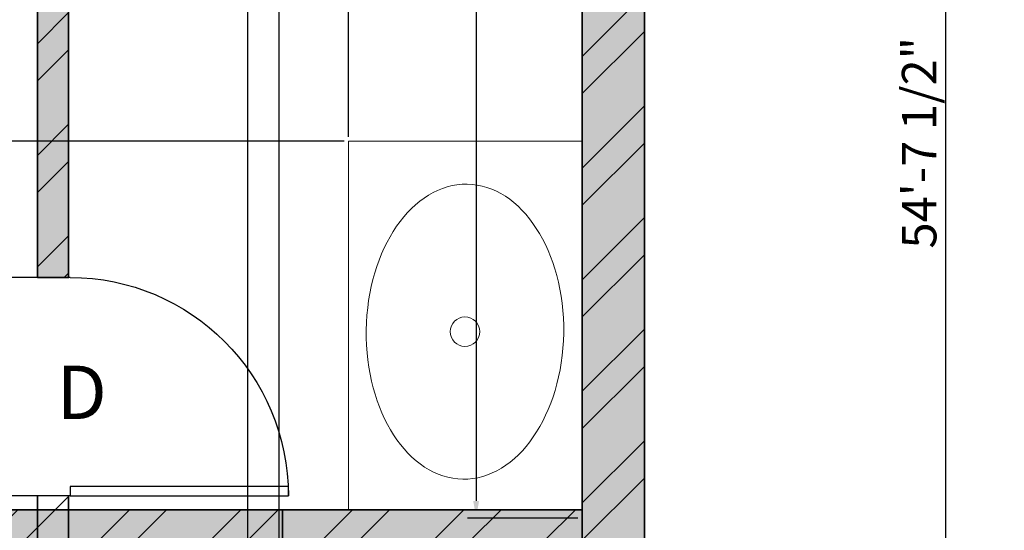
# Model space of a CAD drawing. Units: inches. Extents: x 1804 to 3296, y 909 to 2477.
# Tile 15 of 31: x 2235 to 2378, y 1410 to 1484. Entities that reach past the tile are written whole.
import ezdxf

# ---------------------------------------------------------------- set-up
doc = ezdxf.new("R2010")
doc.units = ezdxf.units.IN
for name, color, linetype, lineweight in [('A-ANNO-DIMS', 2, 'Continuous', 18), ('A-ANNO-TTLB', 156, 'Continuous', 35), ('A-FLOR-FIXT', 9, 'Continuous', 18), ('A-WALL-PATT', 10, 'Continuous', 13), ('DOOR', 30, 'Continuous', 25), ('TEXT', 190, 'Continuous', 18), ('WALL', 10, 'Continuous', 35)]:
    doc.layers.add(name, color=color, linetype=linetype, lineweight=lineweight)
doc.styles.get("Standard").update_dxf_attribs({"font": 'arial.ttf'})
doc.dimstyles.new('ISO-25', dxfattribs={"dimtxt": 5, "dimasz": 2.5, "dimexe": 1.25, "dimexo": 0.625, "dimtad": 1, "dimdec": 0, "dimlunit": 4, "dimtxsty": 'Standard', "dimcen": 2.5, "dimadec": 0, "dimazin": 0, "dimtfac": 1, "dimtdec": 0, "dimtmove": 0, "dimatfit": 3, "dimfxl": 1, "dimarcsym": 0})

# ---------------------------------------------------------------- blocks, each defined once
blk = doc.blocks.new('*U2')
for p, q in [((0, 0), (0, -6)), ((40, 0), (40, -6))]:
    blk.add_line(p, q)
blk.add_lwpolyline([(0, 0), (0, 40), (1.75, 40), (1.75, 0)], close=True)
blk.add_arc((0, 0), 40, 0, 90)
blk = doc.blocks.new('*D13')
at = {"layer": 'A-ANNO-DIMS', "color": 0, "lineweight": -2, "transparency": 16777216}
for p, q in [((2315.91, 1586.42), (2299.9, 1586.42)), ((2301.15, 1583.92), (2301.15, 1413.85)), ((2315.91, 1411.35), (2299.9, 1411.35))]:
    blk.add_line(p, q, dxfattribs=at)
at = {"layer": 'A-ANNO-DIMS', "color": 0, "lineweight": 100, "transparency": 16777216}
for points in [[(2300.73, 1583.92), (2301.57, 1583.92), (2301.15, 1586.42)], [(2300.73, 1413.85), (2301.57, 1413.85), (2301.15, 1411.35)]]:
    blk.add_solid(points, dxfattribs=at)
at = {"layer": 'Defpoints', "color": 0, "lineweight": 100, "transparency": 16777216}
for p in [(2316.54, 1586.42), (2301.15, 1411.35), (2316.54, 1411.35)]:
    blk.add_point(p, dxfattribs=at)
at = {"layer": 'A-ANNO-DIMS', "color": 0, "transparency": 16777216, "insert": (2298.02, 1498.89), "char_height": 5, "attachment_point": 5, "rotation": 90}
blk.add_mtext('14\'-7"', dxfattribs=at)
blk = doc.blocks.new('*D53')
at = {"layer": 'A-ANNO-DIMS', "color": 0, "lineweight": -2, "transparency": 16777216}
for p, q in [((2326.16, 1793.38), (2370.49, 1793.38)), ((2369.24, 1140.57), (2369.24, 1790.88)), ((2326.16, 1138.07), (2370.49, 1138.07))]:
    blk.add_line(p, q, dxfattribs=at)
at = {"layer": 'A-ANNO-DIMS', "color": 0, "lineweight": 100, "transparency": 16777216}
for points in [[(2368.82, 1790.88), (2369.65, 1790.88), (2369.24, 1793.38)], [(2368.82, 1140.57), (2369.65, 1140.57), (2369.24, 1138.07)]]:
    blk.add_solid(points, dxfattribs=at)
at = {"layer": 'Defpoints', "color": 0, "lineweight": 100, "transparency": 16777216}
for p in [(2325.54, 1793.38), (2369.24, 1793.38), (2325.54, 1138.07)]:
    blk.add_point(p, dxfattribs=at)
at = {"layer": 'A-ANNO-DIMS', "color": 0, "transparency": 16777216, "insert": (2366.03, 1465.72), "char_height": 5, "attachment_point": 5, "rotation": 90}
blk.add_mtext('54\'-7 1/2"', dxfattribs=at)
blk = doc.blocks.new('*D56')
at = {"layer": 'A-ANNO-DIMS', "color": 0, "lineweight": -2, "transparency": 16777216}
for p, q in [((2180.87, 1680.42), (2180.87, 975.89)), ((2268, 1680.42), (2268, 975.89)), ((2183.37, 977.14), (2265.5, 977.14))]:
    blk.add_line(p, q, dxfattribs=at)
at = {"layer": 'A-ANNO-DIMS', "color": 0, "lineweight": 100, "transparency": 16777216}
for points in [[(2183.37, 977.56), (2183.37, 976.72), (2180.87, 977.14)], [(2265.5, 977.56), (2265.5, 976.72), (2268, 977.14)]]:
    blk.add_solid(points, dxfattribs=at)
at = {"layer": 'Defpoints', "color": 0, "lineweight": 100, "transparency": 16777216}
for p in [(2180.87, 1681.04), (2268, 1681.04), (2268, 977.14)]:
    blk.add_point(p, dxfattribs=at)
at = {"layer": 'A-ANNO-DIMS', "color": 0, "transparency": 16777216, "insert": (2224.44, 980.32), "char_height": 5, "attachment_point": 5}
blk.add_mtext('7\'-3"', dxfattribs=at)
blk = doc.blocks.new('*D64')
at = {"layer": 'A-ANNO-DIMS', "color": 0, "lineweight": -2, "transparency": 16777216}
for p, q in [((2241.43, 1446.21), (1880.63, 1446.21)), ((1881.88, 1417.08), (1881.88, 1443.71)), ((2241.43, 1414.58), (1880.63, 1414.58))]:
    blk.add_line(p, q, dxfattribs=at)
at = {"layer": 'A-ANNO-DIMS', "color": 0, "lineweight": 100, "transparency": 16777216}
for points in [[(1881.47, 1443.71), (1882.3, 1443.71), (1881.88, 1446.21)], [(1881.47, 1417.08), (1882.3, 1417.08), (1881.88, 1414.58)]]:
    blk.add_solid(points, dxfattribs=at)
at = {"layer": 'Defpoints', "color": 0, "lineweight": 100, "transparency": 16777216}
for p in [(1881.88, 1446.21), (2242.06, 1446.21), (2242.06, 1414.58)]:
    blk.add_point(p, dxfattribs=at)
at = {"layer": 'A-ANNO-DIMS', "color": 0, "transparency": 16777216, "insert": (1878.67, 1430.39), "char_height": 5, "attachment_point": 5, "rotation": 90}
blk.add_mtext('2\'-7 1/2"', dxfattribs=at)
blk = doc.blocks.new('*D65')
at = {"layer": 'A-ANNO-DIMS', "color": 0, "lineweight": -2, "transparency": 16777216}
for p, q in [((2282.65, 1466.57), (2282.65, 1874.99)), ((2316.54, 1466.57), (2316.54, 1874.99)), ((2285.15, 1873.74), (2314.04, 1873.74))]:
    blk.add_line(p, q, dxfattribs=at)
at = {"layer": 'A-ANNO-DIMS', "color": 0, "lineweight": 100, "transparency": 16777216}
for points in [[(2285.15, 1874.15), (2285.15, 1873.32), (2282.65, 1873.74)], [(2314.04, 1874.15), (2314.04, 1873.32), (2316.54, 1873.74)]]:
    blk.add_solid(points, dxfattribs=at)
at = {"layer": 'Defpoints', "color": 0, "lineweight": 100, "transparency": 16777216}
for p in [(2316.54, 1873.74), (2282.65, 1465.94), (2316.54, 1465.94)]:
    blk.add_point(p, dxfattribs=at)
at = {"layer": 'A-ANNO-DIMS', "color": 0, "transparency": 16777216, "insert": (2299.6, 1876.91), "char_height": 5, "attachment_point": 5}
blk.add_mtext('2\'-10"', dxfattribs=at)
blk = doc.blocks.new('*D66')
at = {"layer": 'A-ANNO-DIMS', "color": 0, "lineweight": -2, "transparency": 16777216}
for p, q in [((2282.03, 1465.94), (1880.63, 1465.94)), ((1881.88, 1415.06), (1881.88, 1463.44)), ((2282.03, 1412.56), (1880.63, 1412.56))]:
    blk.add_line(p, q, dxfattribs=at)
at = {"layer": 'A-ANNO-DIMS', "color": 0, "lineweight": 100, "transparency": 16777216}
for points in [[(1881.47, 1463.44), (1882.3, 1463.44), (1881.88, 1465.94)], [(1881.47, 1415.06), (1882.3, 1415.06), (1881.88, 1412.56)]]:
    blk.add_solid(points, dxfattribs=at)
at = {"layer": 'Defpoints', "color": 0, "lineweight": 100, "transparency": 16777216}
for p in [(1881.88, 1465.94), (2282.65, 1465.94), (2282.65, 1412.56)]:
    blk.add_point(p, dxfattribs=at)
at = {"layer": 'A-ANNO-DIMS', "color": 0, "transparency": 16777216, "insert": (1878.67, 1439.25), "char_height": 5, "attachment_point": 5, "rotation": 90}
blk.add_mtext('4\'-5 1/2"', dxfattribs=at)
blk = doc.blocks.new('*D73')
at = {"layer": 'A-ANNO-DIMS', "color": 0, "lineweight": -2, "transparency": 16777216}
for p, q in [((2272.59, 1272.26), (2272.59, 1874.99)), ((2316.54, 1272.26), (2316.54, 1874.99)), ((2275.09, 1873.74), (2314.04, 1873.74))]:
    blk.add_line(p, q, dxfattribs=at)
at = {"layer": 'A-ANNO-DIMS', "color": 0, "lineweight": 100, "transparency": 16777216}
for points in [[(2275.09, 1874.15), (2275.09, 1873.32), (2272.59, 1873.74)], [(2314.04, 1874.15), (2314.04, 1873.32), (2316.54, 1873.74)]]:
    blk.add_solid(points, dxfattribs=at)
at = {"layer": 'Defpoints', "color": 0, "lineweight": 100, "transparency": 16777216}
for p in [(2316.54, 1873.74), (2272.59, 1271.63), (2316.54, 1271.63)]:
    blk.add_point(p, dxfattribs=at)
at = {"layer": 'A-ANNO-DIMS', "color": 0, "transparency": 16777216, "insert": (2294.56, 1876.92), "char_height": 5, "attachment_point": 5}
blk.add_mtext('3\'-8"', dxfattribs=at)

msp = doc.modelspace()

# ---------------------------------------------------------------- hatches: boundary and pattern name
at = {"layer": 'A-ANNO-TTLB'}
h = msp.add_hatch(color=256, dxfattribs=at)
h.dxf.hatch_style = 1
h.paths.add_polyline_path([(3294.53, 2476.54), (1803.79, 2476.54), (1805.43, 909.47), (3296.17, 909.47)])
h.paths.add_polyline_path([(1811, 914.33), (1812.79, 2467.54), (3285.53, 2467.54), (3283.74, 914.33)], flags=16)
h.paths.add_polyline_path([(1925.58, 1062.77), (1925.58, 1138.07), (1925.58, 1539.88), (1925.58, 1793.38), (1925.58, 1830.04), (2325.54, 1830.04), (2325.54, 1793.38), (2325.54, 1586.42), (2325.54, 1138.07), (2325.54, 1062.77)], flags=0)
h.paths.add_polyline_path([(1997.22, 1029.4), (2008.85, 1037.96), (2008.85, 1020.84)], flags=0)
h.paths.add_polyline_path([(1934.58, 1138.07), (1934.58, 1147.07), (2078.77, 1147.07), (2078.77, 1138.07), (2060.94, 1138.07)], flags=0)
h.paths.add_polyline_path([(1944.35, 1138.07), (1944.35, 1147.07), (2056.05, 1147.07), (2056.05, 1138.07)], flags=0)
h.paths.add_polyline_path([(2222.24, 1037.96), (2233.87, 1029.4), (2222.24, 1020.84)], flags=0)
h.paths.add_polyline_path([(2061.94, 1139.07), (2061.94, 1146.07), (2077.77, 1146.07), (2077.77, 1139.07)], flags=0)
h.paths.add_polyline_path([(2149.58, 1138.07), (2149.58, 1269.44), (2158.58, 1269.44), (2158.58, 1326.69), (2149.58, 1326.69), (2149.58, 1340.94), (2139.6, 1340.94), (2139.6, 1434.25), (2149.58, 1434.25), (2149.58, 1447.36), (2158.58, 1447.36), (2158.58, 1423.87), (2158.58, 1408.06), (2198.46, 1408.06), (2198.46, 1412.56), (2282.65, 1412.56), (2282.65, 1465.94), (2316.54, 1465.94), (2316.54, 1590.92), (2192.86, 1590.92), (2192.86, 1595.3), (2291.17, 1595.3), (2291.17, 1590.92), (2316.54, 1590.92), (2316.54, 1784.38), (2300.24, 1784.38), (2300.24, 1757.47), (2268, 1757.47), (2268, 1681.04), (2180.87, 1681.04), (2180.87, 1757.47), (2148.63, 1757.47), (2148.63, 1784.38), (2119.08, 1784.38), (2119.08, 1585.58), (2114.58, 1585.58), (2114.58, 1784.38), (2064.11, 1784.38), (2046.28, 1784.38), (2046.28, 1760.38), (1958.58, 1760.38), (1958.58, 1664.38), (1934.58, 1664.38), (1934.58, 1784.38), (1934.58, 1793.38), (2046.28, 1793.38), (2064.11, 1793.38), (2119.08, 1793.38), (2230.78, 1793.38), (2230.78, 1784.38), (2268, 1784.38), (2300.24, 1784.38), (2316.54, 1784.38), (2316.54, 1590.92), (2316.54, 1373.73), (2316.54, 1138.07)], flags=0)
h.paths.add_polyline_path([(2209.19, 1166.63), (2209.19, 1175.63), (2158.58, 1175.63), (2209.19, 1223.63), (2209.19, 1231.63), (2183.88, 1231.63), (2183.88, 1301.66), (2242.59, 1301.66), (2242.59, 1326.69), (2316.54, 1326.69), (2272.59, 1271.63), (2272.59, 1223.63), (2316.54, 1175.63), (2272.59, 1175.63), (2272.59, 1166.63)], flags=0)
h.paths.add_polyline_path([(1947.77, 1345.22), (1947.77, 1457.48), (1991.2, 1457.48), (1991.2, 1451.7), (1991.2, 1352.18), (1991.2, 1345.22)], flags=0)
h.paths.add_polyline_path([(2209.19, 1271.63), (2262.59, 1271.63), (2262.59, 1311.85), (2272.59, 1301.66), (2272.59, 1271.63), (2269.92, 1269.63), (2270.59, 1269.63), (2270.59, 1225.63), (2211.19, 1225.63), (2211.19, 1269.63), (2211.86, 1269.63)], flags=0)
h.paths.add_polyline_path([(2000.34, 1378.21), (2000.34, 1429.71), (2025.22, 1429.71), (2025.22, 1378.21)], flags=0)
h.paths.add_polyline_path([(2001.34, 1379.21), (2001.34, 1428.71), (2024.22, 1428.71), (2024.22, 1379.21)], flags=0)
h.paths.add_polyline_path([(2012.34, 1390.21), (2012.34, 1417.71), (2013.22, 1417.71), (2013.22, 1390.21)], flags=0)
h.paths.add_polyline_path([(2237.56, 1331.19), (2237.56, 1340.18), (2238.62, 1340.18), (2238.62, 1386.84), (2241.04, 1386.84), (2242.06, 1386.84), (2242.06, 1408.06), (2316.54, 1331.19)], flags=0)
h.paths.add_polyline_path([(1953.73, 1464.35), (1953.73, 1498.59), (1981.74, 1498.59), (1981.74, 1464.35)], flags=0)
h.paths.add_polyline_path([(1987.63, 1462.08), (1987.63, 1500.95), (2104.07, 1500.95), (2104.07, 1462.08), (2099.27, 1462.08), (1993.6, 1462.08)], flags=0)
h.paths.add_polyline_path([(1956.06, 1481.47, -1), (1979.41, 1481.47, -1)], flags=0)
edge = h.paths.add_edge_path(flags=0)
edge.add_ellipse((2299.53, 1438.37), major_axis=(0.31, 21.36), ratio=0.670333, start_angle=0, end_angle=360)
h.paths.add_polyline_path([(2297.39, 1438.37, -1), (2301.67, 1438.37, -1)], flags=0)
h.paths.add_polyline_path([(2591.54, 1163.23), (2591.54, 1179.38), (2591.54, 1379.68), (2591.54, 1395.84), (2734.5, 1395.84), (2734.5, 1379.68), (2734.5, 1179.38), (2734.5, 1163.23)], flags=0)
h.paths.add_polyline_path([(2592.54, 1164.23), (2592.54, 1166.23), (2733.5, 1166.23), (2733.5, 1164.23)], flags=0)
h.paths.add_polyline_path([(2592.54, 1180.38), (2592.54, 1378.68), (2733.5, 1378.68), (2733.5, 1180.38)], flags=0)
h.paths.add_polyline_path([(2593.54, 1181.38), (2593.54, 1377.68), (2732.5, 1377.68), (2732.5, 1181.38)], flags=0)
h.paths.add_polyline_path([(2594.54, 1182.38), (2594.54, 1376.68), (2731.5, 1376.68), (2731.5, 1182.38)], flags=0)
h.paths.add_polyline_path([(1936.95, 1697.46), (1936.95, 1736.46), (1955.41, 1736.46), (1955.41, 1697.46)], flags=0)
h.paths.add_polyline_path([(1938.48, 1718.36), (1938.48, 1734.92), (1953.65, 1734.92), (1953.65, 1718.36)], flags=0)
h.paths.add_polyline_path([(1944.75, 1726.64, -1), (1947.37, 1726.64, -1)], flags=0)
h.paths.add_polyline_path([(2592.54, 1394.84), (2733.5, 1394.84), (2733.5, 1392.84), (2592.54, 1392.84)], flags=0)
h.paths.add_polyline_path([(1976.61, 1762.5), (1976.61, 1781.44), (2012.79, 1781.44), (2012.79, 1762.5)], flags=0)
h.paths.add_polyline_path([(1979.57, 1771.97, -1), (1991.39, 1771.97, -1)], flags=0)
h.paths.add_polyline_path([(1995.36, 1771.97, -1), (2007.18, 1771.97, -1)], flags=0)
h.paths.add_polyline_path([(2251.51, 1744.53), (2268, 1730.05), (2251.51, 1730.05)], flags=0)
h.paths.add_polyline_path([(2047.28, 1785.38), (2047.28, 1792.38), (2063.11, 1792.38), (2063.11, 1785.38)], flags=0)
h.paths.add_polyline_path([(2155.08, 1770.92, -1), (2174.42, 1770.92, -1)], flags=0)
h.paths.add_polyline_path([(2188.59, 1758.27), (2188.59, 1772.81), (2222.3, 1772.81), (2222.3, 1758.27)], flags=0)
h.paths.add_polyline_path([(2223.97, 1758.27), (2223.97, 1772.81), (2257.68, 1772.81), (2257.68, 1758.27)], flags=0)
h.paths.add_polyline_path([(2274.45, 1770.92, -1), (2293.8, 1770.92, -1)], flags=0)
h.paths.add_polyline_path([(2591.54, 1582.09), (2591.54, 1782.39), (2734.5, 1782.39), (2734.5, 1582.09)], flags=0)
h.paths.add_polyline_path([(2592.54, 1583.09), (2592.54, 1781.39), (2733.5, 1781.39), (2733.5, 1583.09)], flags=0)
h.paths.add_polyline_path([(2593.54, 1584.09), (2593.54, 1780.39), (2732.5, 1780.39), (2732.5, 1584.09)], flags=0)
h.paths.add_polyline_path([(2594.54, 1585.09), (2594.54, 1779.39), (2731.5, 1779.39), (2731.5, 1585.09)], flags=0)
h.paths.add_polyline_path([(1922.17, 1978.79), (1922.17, 2295.08), (1922.17, 2296.08), (2115.67, 2296.08), (2115.67, 2384.31), (2115.67, 2385.31), (2322.12, 2385.31), (2323.12, 2385.31), (2323.12, 1979.79), (2323.12, 1978.79), (1923.17, 1978.79)], flags=0)
h.paths.add_polyline_path([(1922.17, 1978.79), (1922.17, 2051.31), (1922.17, 2214.86), (1922.17, 2296.08), (2115.67, 2296.08), (2115.67, 2385.31), (2323.12, 2385.31), (2323.12, 2280.42), (2323.12, 1978.79), (2115.67, 1978.79)], flags=0)
h.paths.add_polyline_path([(1923.17, 1979.79), (1923.17, 2050.31), (2115.67, 2050.31), (2115.67, 2051.31), (1923.17, 2051.31), (1923.17, 2213.86), (1923.17, 2214.86), (1923.17, 2295.08), (1990.02, 2295.08), (1990.02, 2214.86), (1991.02, 2214.86), (1991.02, 2295.08), (2115.67, 2295.08), (2115.67, 1979.79), (2116.67, 1979.79), (2116.67, 2304.18), (2116.67, 2384.31), (2322.12, 2384.31), (2322.12, 2280.42), (2322.12, 1979.79), (2115.67, 1979.79)], flags=0)
h.paths.add_polyline_path([(2972.46, 1192.5), (2972.46, 1196.92), (2995.47, 1196.92), (2995.47, 1255.47), (2995.09, 1255.47), (2987.42, 1249.39), (2980.08, 1255.47), (2978.05, 1255.47), (2978.05, 1257.24), (2995.47, 1257.24), (2995.47, 1261.58), (3015.37, 1261.58), (3015.37, 1333.28), (3015.37, 1414.4), (3032.82, 1414.4), (3032.82, 1333.28), (3032.82, 1261.58), (3052.66, 1261.58), (3052.66, 1255.47), (3079.86, 1255.47), (3078.72, 1254.57), (3081.47, 1252.29), (3078.56, 1249.99), (3075.81, 1252.26), (3072.57, 1249.69), (3070.36, 1251.52), (3067.67, 1249.39), (3060.34, 1255.47), (3052.66, 1255.47), (3052.66, 1196.92), (3054.58, 1196.92), (3074, 1196.92), (3074, 1192.5), (3052.66, 1192.5), (2995.47, 1192.5)], flags=0)
h.paths.add_polyline_path([(2490.75, 1979.27), (2490.75, 1980.27), (2596.87, 1980.27), (2596.87, 2051.8), (2596.87, 2052.8), (2596.87, 2216.35), (2596.87, 2297.57), (2717.32, 2297.57), (2710.57, 2305.62), (2724.07, 2305.62), (2717.32, 2297.57), (2782.37, 2297.57), (2782.37, 2395.8), (3006.82, 2395.8), (3006.82, 1981.27), (3093.73, 1981.27), (3093.73, 1980.27), (3047.51, 1980.27), (3046.37, 1979.37), (3049.11, 1977.1), (3046.2, 1974.79), (3043.46, 1977.07), (3040.21, 1974.49), (3038, 1976.32), (3035.32, 1974.2), (3027.98, 1980.27), (2871.83, 1980.27), (2871.83, 1981.27), (2791.37, 1981.27), (2791.37, 2050.8), (2597.87, 2050.8), (2597.87, 1980.27), (2597.87, 1979.27), (2546.27, 1979.27), (2545.12, 1978.37), (2547.87, 1976.1), (2544.96, 1973.79), (2542.22, 1976.07), (2538.97, 1973.49), (2536.76, 1975.32), (2534.07, 1973.2), (2526.74, 1979.27)], flags=0)
h.paths.add_polyline_path([(2597.87, 2051.8), (2606.87, 2051.8), (2606.87, 2258.39), (2597.87, 2258.39), (2597.87, 2296.57), (2606.87, 2296.57), (2606.87, 2262.39), (2782.37, 2262.39), (2782.37, 2296.57), (2790.37, 2296.57), (2790.37, 2262.39), (2791.37, 2262.39), (2791.37, 2305.67), (2791.37, 2385.8), (2996.82, 2385.8), (2996.82, 2339.85), (3006.82, 2339.85), (3006.82, 2250.12), (2997.82, 2250.12), (2997.82, 1981.27), (2996.82, 1981.27), (2872.83, 1981.27), (2872.83, 1991.8), (2871.83, 1991.8), (2871.83, 2050.8), (2790.37, 2050.8), (2597.87, 2050.8)], flags=0)
h.paths.add_polyline_path([(2179.93, 2153.92), (2179.93, 2353.97), (2259.98, 2353.97), (2259.98, 2153.92)], flags=0)
h.paths.add_polyline_path([(2180.93, 2154.92), (2180.93, 2352.97), (2258.98, 2352.97), (2258.98, 2154.92)], flags=0)
h.paths.add_polyline_path([(2960.87, 1608.49), (2960.87, 1753.62), (3070.9, 1753.62), (3070.9, 1608.49)], flags=0)
h.paths.add_polyline_path([(2961.87, 1609.49), (2961.87, 1752.62), (3069.9, 1752.62), (3069.9, 1609.49)], flags=0)
h.paths.add_polyline_path([(2962.87, 1610.49), (2962.87, 1751.62), (3068.9, 1751.62), (3068.9, 1610.49)], flags=0)
h.paths.add_polyline_path([(2963.87, 1611.49), (2963.87, 1750.62), (3067.9, 1750.62), (3067.9, 1611.49)], flags=0)
h.paths.add_polyline_path([(2782.37, 2051.8), (2782.37, 2216.32), (2791.37, 2216.32), (2791.37, 2051.8), (2872.83, 2051.8), (2872.83, 2068.56), (2884.67, 2068.56), (2884.67, 2085.33), (2896.51, 2085.33), (2896.51, 2102.09), (2908.36, 2102.09), (2908.36, 2118.85), (2920.2, 2118.85), (2920.2, 2135.62), (2932.05, 2135.62), (2932.05, 2145.3), (2925.08, 2145.3), (2925.08, 2203.2), (2996.82, 2203.2), (2996.82, 2145.3), (2953.82, 2145.3), (2872.83, 2051.8), (2790.37, 2051.8)], flags=0)
h.paths.add_polyline_path([(2717.32, 2238.65), (2710.57, 2246.7), (2724.07, 2246.7)], flags=0)
h.paths.add_polyline_path([(2003.09, 1122.79), (2017.16, 1122.79), (2017.16, 1138.74), (2003.09, 1138.74)], flags=8)
h.paths.add_polyline_path([(2174.76, 1792.72), (2188.83, 1792.72), (2188.83, 1808.66), (2174.76, 1808.66)], flags=8)
h.paths.add_polyline_path([(1987.95, 1792.51), (2002.02, 1792.51), (2002.02, 1808.45), (1987.95, 1808.45)], flags=8)
h.paths.add_polyline_path([(2148.79, 1289.26), (2160.46, 1289.26), (2160.46, 1305.2), (2148.79, 1305.2)], flags=8)
h.paths.add_polyline_path([(2115.36, 1133.57), (2127.04, 1133.57), (2127.04, 1149.51), (2115.36, 1149.51)], flags=8)
h.paths.add_polyline_path([(2237.58, 1421.48), (2249.25, 1421.48), (2249.25, 1437.43), (2237.58, 1437.43)], flags=8)
h.paths.add_polyline_path([(2134.99, 1584.32), (2146.66, 1584.32), (2146.66, 1600.26), (2134.99, 1600.26)], flags=8)
h.paths.add_polyline_path([(2101.95, 1557.31), (2113.62, 1557.31), (2113.62, 1573.25), (2101.95, 1573.25)], flags=8)
h.paths.add_polyline_path([(2937.85, 1156.77), (3120.41, 1156.77), (3120.41, 1185.72), (2937.85, 1185.72)], flags=8)
h.paths.add_polyline_path([(2980.71, 1786.71), (3050.06, 1786.71), (3050.06, 1802.66), (2980.71, 1802.66)], flags=8)
h.paths.add_polyline_path([(2869.28, 1661.96), (2938.62, 1661.96), (2938.62, 1690.8), (2869.28, 1690.8)], flags=8)
h.paths.add_polyline_path([(3092.27, 1674.86), (3161.62, 1674.86), (3161.62, 1690.8), (3092.27, 1690.8)], flags=8)
h.paths.add_polyline_path([(2980.71, 1674.86), (3050.06, 1674.86), (3050.06, 1690.8), (2980.71, 1690.8)], flags=8)
h.paths.add_polyline_path([(2649.07, 1678.23), (2674.53, 1678.23), (2674.53, 1714.76), (2649.07, 1714.76)], flags=8)
h.paths.add_polyline_path([(2530.84, 1981.63), (2549.13, 1981.63), (2549.13, 1997.57), (2530.84, 1997.57)], flags=8)
h.paths.add_polyline_path([(3031.29, 1981.77), (3049.58, 1981.77), (3049.58, 1997.71), (3031.29, 1997.71)], flags=8)
h.paths.add_polyline_path([(2715.38, 1911.9), (2851.54, 1911.9), (2851.54, 1940.85), (2715.38, 1940.85)], flags=8)
h.paths.add_polyline_path([(2015.23, 1927.36), (2205.42, 1927.36), (2205.42, 1956.3), (2015.23, 1956.3)], flags=8)
h.paths.add_polyline_path([(2671.84, 2057.84), (2702.75, 2057.84), (2702.75, 2073.79), (2671.84, 2073.79)], flags=8)
h.paths.add_polyline_path([(2678.5, 2316.52), (2765.26, 2316.52), (2765.26, 2332.46), (2678.5, 2332.46)], flags=8)
h.paths.add_polyline_path([(2678.48, 2271.96), (2736.41, 2271.96), (2736.41, 2287.9), (2678.48, 2287.9)], flags=8)
h.paths.add_polyline_path([(2019.2, 972.79), (2243.21, 972.79), (2243.21, 1001.74), (2019.2, 1001.74)], flags=8)
h.paths.add_polyline_path([(2097.06, 1021.56), (2132.16, 1021.56), (2132.16, 1037.51), (2097.06, 1037.51)], flags=8)
h.paths.add_polyline_path([(2182.47, 1360.48), (2207.35, 1360.48), (2207.35, 1376.42), (2182.47, 1376.42)], flags=8)
h.paths.add_polyline_path([(2261.12, 1361.77), (2295.01, 1361.77), (2295.01, 1377.71), (2261.12, 1377.71)], flags=8)
h.paths.add_polyline_path([(2245.75, 1511.51), (2278.44, 1511.51), (2278.44, 1527.46), (2245.75, 1527.46)], flags=8)
h.paths.add_polyline_path([(1991.16, 1296.29), (2060.51, 1296.29), (2060.51, 1312.23), (1991.16, 1312.23)], flags=8)
h.paths.add_polyline_path([(2187, 1651.35), (2246.71, 1651.35), (2246.71, 1667.29), (2187, 1667.29)], flags=8)
h.paths.add_polyline_path([(1976.49, 1684.81), (2068.63, 1684.81), (2068.63, 1700.76), (1976.49, 1700.76)], flags=8)
at = {"layer": 'A-WALL-PATT'}
h = msp.add_hatch(color=256, dxfattribs=at)
h.dxf.hatch_style = 1
h.paths.add_polyline_path([(2119.08, 1544.38), (1925.58, 1544.38), (1925.58, 1539.88), (2119.08, 1539.88)])
h.paths.add_polyline_path([(2119.08, 1545.58), (2114.58, 1545.58), (2114.58, 1544.38), (2119.08, 1544.38)])
h.paths.add_polyline_path([(1965.87, 1658.79), (1965.87, 1679.09), (1955.57, 1679.09), (1955.57, 1658.79)], flags=9)
h.paths.add_polyline_path([(2293.18, 1677.29), (2293.18, 1697.58), (2282.88, 1697.58), (2282.88, 1677.29)], flags=9)
h.paths.add_polyline_path([(2271.13, 1545.23), (2287.53, 1545.23), (2287.53, 1555.53), (2271.13, 1555.53)], flags=9)
h.paths.add_polyline_path([(2303.26, 1488.52), (2303.26, 1508.82), (2292.95, 1508.82), (2292.95, 1488.52)], flags=9)
h.paths.add_polyline_path([(2271.13, 1393.15), (2287.53, 1393.15), (2287.53, 1403.45), (2271.13, 1403.45)], flags=9)
h.paths.add_polyline_path([(2306.48, 1361.45), (2306.48, 1377.86), (2296.18, 1377.86), (2296.18, 1361.45)], flags=9)
h.paths.add_polyline_path([(2174.54, 1361.45), (2174.54, 1377.86), (2164.23, 1377.86), (2164.23, 1361.45)], flags=9)
h.paths.add_polyline_path([(1968.21, 1333.34), (1968.21, 1353.64), (1957.91, 1353.64), (1957.91, 1333.34)], flags=9)
h.paths.add_polyline_path([(2003.09, 1122.79), (2017.16, 1122.79), (2017.16, 1138.74), (2003.09, 1138.74)], flags=9)
h.paths.add_polyline_path([(2174.76, 1792.72), (2188.83, 1792.72), (2188.83, 1808.66), (2174.76, 1808.66)], flags=9)
h.paths.add_polyline_path([(1987.95, 1792.51), (2002.02, 1792.51), (2002.02, 1808.45), (1987.95, 1808.45)], flags=9)
h.paths.add_polyline_path([(2148.79, 1289.26), (2160.46, 1289.26), (2160.46, 1305.2), (2148.79, 1305.2)], flags=9)
h.paths.add_polyline_path([(2115.36, 1133.57), (2127.04, 1133.57), (2127.04, 1149.51), (2115.36, 1149.51)], flags=9)
h.paths.add_polyline_path([(2237.58, 1421.48), (2249.25, 1421.48), (2249.25, 1437.43), (2237.58, 1437.43)], flags=9)
h.paths.add_polyline_path([(2134.99, 1584.32), (2146.66, 1584.32), (2146.66, 1600.26), (2134.99, 1600.26)], flags=9)
h.paths.add_polyline_path([(2101.95, 1557.31), (2113.62, 1557.31), (2113.62, 1573.25), (2101.95, 1573.25)], flags=9)
h.paths.add_polyline_path([(2937.85, 1156.77), (3120.41, 1156.77), (3120.41, 1185.72), (2937.85, 1185.72)], flags=9)
h.paths.add_polyline_path([(2980.71, 1786.71), (3050.06, 1786.71), (3050.06, 1802.66), (2980.71, 1802.66)], flags=9)
h.paths.add_polyline_path([(2869.28, 1661.96), (2938.62, 1661.96), (2938.62, 1690.8), (2869.28, 1690.8)], flags=9)
h.paths.add_polyline_path([(3092.27, 1674.86), (3161.62, 1674.86), (3161.62, 1690.8), (3092.27, 1690.8)], flags=9)
h.paths.add_polyline_path([(2980.71, 1674.86), (3050.06, 1674.86), (3050.06, 1690.8), (2980.71, 1690.8)], flags=9)
h.paths.add_polyline_path([(2649.07, 1678.23), (2674.53, 1678.23), (2674.53, 1714.76), (2649.07, 1714.76)], flags=9)
h.paths.add_polyline_path([(2530.84, 1981.63), (2549.13, 1981.63), (2549.13, 1997.57), (2530.84, 1997.57)], flags=9)
h.paths.add_polyline_path([(3031.29, 1981.77), (3049.58, 1981.77), (3049.58, 1997.71), (3031.29, 1997.71)], flags=9)
h.paths.add_polyline_path([(2715.38, 1911.9), (2851.54, 1911.9), (2851.54, 1940.85), (2715.38, 1940.85)], flags=9)
h.paths.add_polyline_path([(2015.23, 1927.36), (2205.42, 1927.36), (2205.42, 1956.3), (2015.23, 1956.3)], flags=9)
h.paths.add_polyline_path([(2671.84, 2057.84), (2702.75, 2057.84), (2702.75, 2073.79), (2671.84, 2073.79)], flags=9)
h.paths.add_polyline_path([(2678.5, 2316.52), (2765.26, 2316.52), (2765.26, 2332.46), (2678.5, 2332.46)], flags=9)
h.paths.add_polyline_path([(2678.48, 2271.96), (2736.41, 2271.96), (2736.41, 2287.9), (2678.48, 2287.9)], flags=9)
h.paths.add_polyline_path([(2019.2, 972.79), (2243.21, 972.79), (2243.21, 1001.74), (2019.2, 1001.74)], flags=9)
h.paths.add_polyline_path([(2097.06, 1021.56), (2132.16, 1021.56), (2132.16, 1037.51), (2097.06, 1037.51)], flags=9)
h.paths.add_polyline_path([(2182.47, 1360.48), (2207.35, 1360.48), (2207.35, 1376.42), (2182.47, 1376.42)], flags=9)
h.paths.add_polyline_path([(2261.12, 1361.77), (2295.01, 1361.77), (2295.01, 1377.71), (2261.12, 1377.71)], flags=9)
h.paths.add_polyline_path([(2245.75, 1511.51), (2278.44, 1511.51), (2278.44, 1527.46), (2245.75, 1527.46)], flags=9)
h.paths.add_polyline_path([(1991.16, 1296.29), (2060.51, 1296.29), (2060.51, 1312.23), (1991.16, 1312.23)], flags=9)
h.paths.add_polyline_path([(2187, 1651.35), (2246.71, 1651.35), (2246.71, 1667.29), (2187, 1667.29)], flags=9)
h.paths.add_polyline_path([(1976.49, 1684.81), (2068.63, 1684.81), (2068.63, 1700.76), (1976.49, 1700.76)], flags=9)
h = msp.add_hatch(color=256, dxfattribs=at)
h.dxf.hatch_style = 1
h.paths.add_polyline_path([(2149.58, 1147.07), (2141.21, 1147.07), (2141.21, 1144.07), (2141.21, 1138.07), (2149.58, 1138.07)])
h.paths.add_polyline_path([(2101.21, 1144.07, -0.01877), (2101.32, 1147.07), (2078.77, 1147.07), (2078.77, 1138.07), (2101.21, 1138.07)])
h.paths.add_polyline_path([(2060.94, 1147.07), (2056.05, 1147.07), (2056.05, 1138.07), (2060.94, 1138.07)])
h.paths.add_polyline_path([(1944.35, 1147.07), (1934.58, 1147.07), (1934.58, 1138.07), (1944.35, 1138.07)])
h.paths.add_polyline_path([(2158.58, 1269.44), (2149.58, 1269.44), (2149.58, 1138.07), (2158.58, 1138.07)])
h.paths.add_polyline_path([(2003.09, 1122.79), (2017.16, 1122.79), (2017.16, 1138.74), (2003.09, 1138.74)], flags=9)
h.paths.add_polyline_path([(2174.76, 1792.72), (2188.83, 1792.72), (2188.83, 1808.66), (2174.76, 1808.66)], flags=9)
h.paths.add_polyline_path([(1987.95, 1792.51), (2002.02, 1792.51), (2002.02, 1808.45), (1987.95, 1808.45)], flags=9)
h.paths.add_polyline_path([(2148.79, 1289.26), (2160.46, 1289.26), (2160.46, 1305.2), (2148.79, 1305.2)], flags=9)
h.paths.add_polyline_path([(2115.36, 1133.57), (2127.04, 1133.57), (2127.04, 1149.51), (2115.36, 1149.51)], flags=9)
h.paths.add_polyline_path([(2237.58, 1421.48), (2249.25, 1421.48), (2249.25, 1437.43), (2237.58, 1437.43)], flags=9)
h.paths.add_polyline_path([(2134.99, 1584.32), (2146.66, 1584.32), (2146.66, 1600.26), (2134.99, 1600.26)], flags=9)
h.paths.add_polyline_path([(2101.95, 1557.31), (2113.62, 1557.31), (2113.62, 1573.25), (2101.95, 1573.25)], flags=9)
h.paths.add_polyline_path([(2937.85, 1156.77), (3120.41, 1156.77), (3120.41, 1185.72), (2937.85, 1185.72)], flags=9)
h.paths.add_polyline_path([(2980.71, 1786.71), (3050.06, 1786.71), (3050.06, 1802.66), (2980.71, 1802.66)], flags=9)
h.paths.add_polyline_path([(2869.28, 1661.96), (2938.62, 1661.96), (2938.62, 1690.8), (2869.28, 1690.8)], flags=9)
h.paths.add_polyline_path([(3092.27, 1674.86), (3161.62, 1674.86), (3161.62, 1690.8), (3092.27, 1690.8)], flags=9)
h.paths.add_polyline_path([(2980.71, 1674.86), (3050.06, 1674.86), (3050.06, 1690.8), (2980.71, 1690.8)], flags=9)
h.paths.add_polyline_path([(2649.07, 1678.23), (2674.53, 1678.23), (2674.53, 1714.76), (2649.07, 1714.76)], flags=9)
h.paths.add_polyline_path([(2530.84, 1981.63), (2549.13, 1981.63), (2549.13, 1997.57), (2530.84, 1997.57)], flags=9)
h.paths.add_polyline_path([(3031.29, 1981.77), (3049.58, 1981.77), (3049.58, 1997.71), (3031.29, 1997.71)], flags=9)
h.paths.add_polyline_path([(2715.38, 1911.9), (2851.54, 1911.9), (2851.54, 1940.85), (2715.38, 1940.85)], flags=9)
h.paths.add_polyline_path([(2015.23, 1927.36), (2205.42, 1927.36), (2205.42, 1956.3), (2015.23, 1956.3)], flags=9)
h.paths.add_polyline_path([(2671.84, 2057.84), (2702.75, 2057.84), (2702.75, 2073.79), (2671.84, 2073.79)], flags=9)
h.paths.add_polyline_path([(2678.5, 2316.52), (2765.26, 2316.52), (2765.26, 2332.46), (2678.5, 2332.46)], flags=9)
h.paths.add_polyline_path([(2678.48, 2271.96), (2736.41, 2271.96), (2736.41, 2287.9), (2678.48, 2287.9)], flags=9)
h.paths.add_polyline_path([(2019.2, 972.79), (2243.21, 972.79), (2243.21, 1001.74), (2019.2, 1001.74)], flags=9)
h.paths.add_polyline_path([(2097.06, 1021.56), (2132.16, 1021.56), (2132.16, 1037.51), (2097.06, 1037.51)], flags=9)
h.paths.add_polyline_path([(2182.47, 1360.48), (2207.35, 1360.48), (2207.35, 1376.42), (2182.47, 1376.42)], flags=9)
h.paths.add_polyline_path([(2261.12, 1361.77), (2295.01, 1361.77), (2295.01, 1377.71), (2261.12, 1377.71)], flags=9)
h.paths.add_polyline_path([(2245.75, 1511.51), (2278.44, 1511.51), (2278.44, 1527.46), (2245.75, 1527.46)], flags=9)
h.paths.add_polyline_path([(1991.16, 1296.29), (2060.51, 1296.29), (2060.51, 1312.23), (1991.16, 1312.23)], flags=9)
h.paths.add_polyline_path([(2187, 1651.35), (2246.71, 1651.35), (2246.71, 1667.29), (2187, 1667.29)], flags=9)
h.paths.add_polyline_path([(1976.49, 1684.81), (2068.63, 1684.81), (2068.63, 1700.76), (1976.49, 1700.76)], flags=9)
h = msp.add_hatch(color=256, dxfattribs=at)
h.dxf.hatch_style = 1
h.paths.add_polyline_path([(2158.58, 1275.49), (2155.29, 1275.49), (2149.58, 1275.49), (2149.58, 1269.44), (2158.58, 1269.44)])
h.paths.add_polyline_path([(2158.58, 1326.69), (2149.58, 1326.69), (2149.58, 1319.33), (2155.29, 1319.33), (2158.58, 1319.33)])
h.paths.add_polyline_path([(2158.58, 1402.2), (2158.58, 1423.87), (2158.58, 1447.36), (2149.58, 1447.36), (2149.58, 1423.87), (2149.58, 1340.94), (2149.58, 1326.69), (2158.58, 1326.69), (2158.58, 1354.23)])
h.paths.add_polyline_path([(1965.87, 1658.79), (1965.87, 1679.09), (1955.57, 1679.09), (1955.57, 1658.79)], flags=9)
h.paths.add_polyline_path([(2293.18, 1677.29), (2293.18, 1697.58), (2282.88, 1697.58), (2282.88, 1677.29)], flags=9)
h.paths.add_polyline_path([(2271.13, 1545.23), (2287.53, 1545.23), (2287.53, 1555.53), (2271.13, 1555.53)], flags=9)
h.paths.add_polyline_path([(2303.26, 1488.52), (2303.26, 1508.82), (2292.95, 1508.82), (2292.95, 1488.52)], flags=9)
h.paths.add_polyline_path([(2271.13, 1393.15), (2287.53, 1393.15), (2287.53, 1403.45), (2271.13, 1403.45)], flags=9)
h.paths.add_polyline_path([(2306.48, 1361.45), (2306.48, 1377.86), (2296.18, 1377.86), (2296.18, 1361.45)], flags=9)
h.paths.add_polyline_path([(2189.9, 1340.62), (2206.31, 1340.62), (2206.31, 1350.92), (2189.9, 1350.92)], flags=9)
h.paths.add_polyline_path([(2174.54, 1361.45), (2174.54, 1377.86), (2164.23, 1377.86), (2164.23, 1361.45)], flags=9)
h.paths.add_polyline_path([(2304.24, 1240.8), (2304.24, 1261.09), (2293.94, 1261.09), (2293.94, 1240.8)], flags=9)
h.paths.add_polyline_path([(2227.19, 1188.73), (2247.49, 1188.73), (2247.49, 1199.03), (2227.19, 1199.03)], flags=9)
h.paths.add_polyline_path([(2181.93, 1144.21), (2181.93, 1160.62), (2171.63, 1160.62), (2171.63, 1144.21)], flags=9)
h.paths.add_polyline_path([(1968.21, 1333.34), (1968.21, 1353.64), (1957.91, 1353.64), (1957.91, 1333.34)], flags=9)
h.paths.add_polyline_path([(2029.78, 1203.53), (2053.95, 1203.53), (2053.95, 1213.83), (2029.78, 1213.83)], flags=9)
h.paths.add_polyline_path([(2576.51, 1671.88), (2576.51, 1692.17), (2566.21, 1692.17), (2566.21, 1671.88)], flags=9)
h.paths.add_polyline_path([(2566.99, 1269.67), (2566.99, 1289.96), (2556.68, 1289.96), (2556.68, 1269.67)], flags=9)
h.paths.add_polyline_path([(2581.85, 1269.17), (2581.85, 1289.46), (2571.54, 1289.46), (2571.54, 1269.17)], flags=9)
h.paths.add_polyline_path([(2650.71, 1409.75), (2674.89, 1409.75), (2674.89, 1420.05), (2650.71, 1420.05)], flags=9)
h.paths.add_polyline_path([(2003.09, 1122.79), (2017.16, 1122.79), (2017.16, 1138.74), (2003.09, 1138.74)], flags=9)
h.paths.add_polyline_path([(2174.76, 1792.72), (2188.83, 1792.72), (2188.83, 1808.66), (2174.76, 1808.66)], flags=9)
h.paths.add_polyline_path([(1987.95, 1792.51), (2002.02, 1792.51), (2002.02, 1808.45), (1987.95, 1808.45)], flags=9)
h.paths.add_polyline_path([(2148.79, 1289.26), (2160.46, 1289.26), (2160.46, 1305.2), (2148.79, 1305.2)], flags=9)
h.paths.add_polyline_path([(2115.36, 1133.57), (2127.04, 1133.57), (2127.04, 1149.51), (2115.36, 1149.51)], flags=9)
h.paths.add_polyline_path([(2237.58, 1421.48), (2249.25, 1421.48), (2249.25, 1437.43), (2237.58, 1437.43)], flags=9)
h.paths.add_polyline_path([(2134.99, 1584.32), (2146.66, 1584.32), (2146.66, 1600.26), (2134.99, 1600.26)], flags=9)
h.paths.add_polyline_path([(2101.95, 1557.31), (2113.62, 1557.31), (2113.62, 1573.25), (2101.95, 1573.25)], flags=9)
h.paths.add_polyline_path([(2937.85, 1156.77), (3120.41, 1156.77), (3120.41, 1185.72), (2937.85, 1185.72)], flags=9)
h.paths.add_polyline_path([(2980.71, 1786.71), (3050.06, 1786.71), (3050.06, 1802.66), (2980.71, 1802.66)], flags=9)
h.paths.add_polyline_path([(2869.28, 1661.96), (2938.62, 1661.96), (2938.62, 1690.8), (2869.28, 1690.8)], flags=9)
h.paths.add_polyline_path([(3092.27, 1674.86), (3161.62, 1674.86), (3161.62, 1690.8), (3092.27, 1690.8)], flags=9)
h.paths.add_polyline_path([(2980.71, 1674.86), (3050.06, 1674.86), (3050.06, 1690.8), (2980.71, 1690.8)], flags=9)
h.paths.add_polyline_path([(2649.07, 1678.23), (2674.53, 1678.23), (2674.53, 1714.76), (2649.07, 1714.76)], flags=9)
h.paths.add_polyline_path([(2530.84, 1981.63), (2549.13, 1981.63), (2549.13, 1997.57), (2530.84, 1997.57)], flags=9)
h.paths.add_polyline_path([(3031.29, 1981.77), (3049.58, 1981.77), (3049.58, 1997.71), (3031.29, 1997.71)], flags=9)
h.paths.add_polyline_path([(2715.38, 1911.9), (2851.54, 1911.9), (2851.54, 1940.85), (2715.38, 1940.85)], flags=9)
h.paths.add_polyline_path([(2015.23, 1927.36), (2205.42, 1927.36), (2205.42, 1956.3), (2015.23, 1956.3)], flags=9)
h.paths.add_polyline_path([(2671.84, 2057.84), (2702.75, 2057.84), (2702.75, 2073.79), (2671.84, 2073.79)], flags=9)
h.paths.add_polyline_path([(2678.5, 2316.52), (2765.26, 2316.52), (2765.26, 2332.46), (2678.5, 2332.46)], flags=9)
h.paths.add_polyline_path([(2678.48, 2271.96), (2736.41, 2271.96), (2736.41, 2287.9), (2678.48, 2287.9)], flags=9)
h.paths.add_polyline_path([(2019.2, 972.79), (2243.21, 972.79), (2243.21, 1001.74), (2019.2, 1001.74)], flags=9)
h.paths.add_polyline_path([(2097.06, 1021.56), (2132.16, 1021.56), (2132.16, 1037.51), (2097.06, 1037.51)], flags=9)
h.paths.add_polyline_path([(2182.47, 1360.48), (2207.35, 1360.48), (2207.35, 1376.42), (2182.47, 1376.42)], flags=9)
h.paths.add_polyline_path([(2261.12, 1361.77), (2295.01, 1361.77), (2295.01, 1377.71), (2261.12, 1377.71)], flags=9)
h.paths.add_polyline_path([(2245.75, 1511.51), (2278.44, 1511.51), (2278.44, 1527.46), (2245.75, 1527.46)], flags=9)
h.paths.add_polyline_path([(1991.16, 1296.29), (2060.51, 1296.29), (2060.51, 1312.23), (1991.16, 1312.23)], flags=9)
h.paths.add_polyline_path([(2187, 1651.35), (2246.71, 1651.35), (2246.71, 1667.29), (2187, 1667.29)], flags=9)
h.paths.add_polyline_path([(1976.49, 1684.81), (2068.63, 1684.81), (2068.63, 1700.76), (1976.49, 1700.76)], flags=9)
h = msp.add_hatch(dxfattribs=at)
h.set_pattern_fill('ANSI32', color=256, scale=1.2)
h.set_pattern_definition([(45, (0, 196.207), (-8.08223, 8.08223), []), (45, (5.388, 196.207), (-8.08223, 8.08223), [])])
h.paths.add_polyline_path([(1934.58, 1784.38), (1934.58, 1793.38), (1925.58, 1793.38), (1925.58, 1539.88), (2119.08, 1539.88), (2119.08, 1545.58), (2114.58, 1545.58), (2114.58, 1544.38), (1934.58, 1544.38)])
h.paths.add_polyline_path([(2114.58, 1793.38), (2064.11, 1793.38), (2064.11, 1784.38), (2114.58, 1784.38)], flags=17)
h.paths.add_polyline_path([(2325.54, 1793.38), (2230.78, 1793.38), (2230.78, 1784.38), (2268, 1784.38), (2300.24, 1784.38), (2316.54, 1784.38), (2316.54, 1590.92), (2316.54, 1586.42), (2325.54, 1586.42)])
h.paths.add_polyline_path([(1944.35, 1147.07), (1934.58, 1147.07), (1934.58, 1138.07), (1944.35, 1138.07)])
h.paths.add_polyline_path([(2101.21, 1144.07, -0.01877), (2101.32, 1147.07), (2078.77, 1147.07), (2078.77, 1138.07), (2101.21, 1138.07)])
h.paths.add_polyline_path([(1934.58, 1539.88), (1925.58, 1539.88), (1925.58, 1138.07), (1934.58, 1138.07), (1934.58, 1147.07)])
h.paths.add_polyline_path([(2325.54, 1586.42), (2316.54, 1586.42), (2316.54, 1373.73), (2316.54, 1138.07), (2325.54, 1138.07), (2325.54, 1228.97)])
h.paths.add_polyline_path([(2158.58, 1423.87), (2158.58, 1447.36), (2149.58, 1447.36), (2149.58, 1423.87), (2149.58, 1340.94), (2149.58, 1326.69), (2158.58, 1326.69), (2158.58, 1354.23), (2158.58, 1402.2)])
h.paths.add_polyline_path([(2316.54, 1412.56), (2282.65, 1412.56), (2273.09, 1412.56), (2273.09, 1408.06), (2316.54, 1408.06)])
h.paths.add_polyline_path([(2273.09, 1412.56), (2242.06, 1412.56), (2242.06, 1408.06), (2273.09, 1408.06)])
h.paths.add_polyline_path([(2237.56, 1412.56), (2198.46, 1412.56), (2198.46, 1408.06), (2237.56, 1408.06)])
h.paths.add_polyline_path([(2242.06, 1408.06), (2237.56, 1408.06), (2237.56, 1386.84), (2242.06, 1386.84)])
h.paths.add_polyline_path([(2242.06, 1412.56), (2237.56, 1412.56), (2237.56, 1408.06), (2242.06, 1408.06)])
h.paths.add_polyline_path([(2158.58, 1269.44), (2149.58, 1269.44), (2149.58, 1138.07), (2158.58, 1138.07)])
h.paths.add_polyline_path([(2149.58, 1147.07), (2141.21, 1147.07), (2141.21, 1144.07), (2141.21, 1138.07), (2149.58, 1138.07)])
h.paths.add_polyline_path([(2272.59, 1175.63), (2209.19, 1175.63), (2209.19, 1166.63), (2272.59, 1166.63)])
h.paths.add_polyline_path([(2237.56, 1446.21), (2242.06, 1446.21), (2242.06, 1586.42), (2237.56, 1586.42)])
h.paths.add_polyline_path([(2242.06, 1414.58), (2237.56, 1414.58), (2237.56, 1412.56), (2242.06, 1412.56)])
h = msp.add_hatch(color=256, dxfattribs=at)
h.dxf.hatch_style = 1
h.paths.add_polyline_path([(2114.58, 1793.38), (2064.11, 1793.38), (2064.11, 1784.38), (2114.58, 1784.38)])
h.paths.add_polyline_path([(2119.08, 1793.38), (2114.58, 1793.38), (2114.58, 1585.58), (2119.08, 1585.58)])
h.paths.add_polyline_path([(2325.54, 1793.38), (2230.78, 1793.38), (2230.78, 1784.38), (2268, 1784.38), (2316.54, 1784.38), (2316.54, 1590.92), (2316.54, 1586.42), (2325.54, 1586.42)])
h.paths.add_polyline_path([(2316.54, 1331.19), (2158.58, 1331.19), (2158.58, 1326.69), (2316.54, 1326.69)])
h.paths.add_polyline_path([(2242.06, 1408.06), (2237.56, 1408.06), (2237.56, 1386.84), (2242.06, 1386.84)])
h.paths.add_polyline_path([(2242.06, 1412.56), (2237.56, 1412.56), (2237.56, 1408.06), (2242.06, 1408.06)])
h.paths.add_polyline_path([(2237.56, 1412.56), (2198.46, 1412.56), (2198.46, 1408.06), (2237.56, 1408.06)])
h.paths.add_polyline_path([(2273.09, 1412.56), (2242.06, 1412.56), (2242.06, 1408.06), (2273.09, 1408.06)])
h.paths.add_polyline_path([(2316.54, 1412.56), (2282.65, 1412.56), (2273.09, 1412.56), (2273.09, 1408.06), (2316.54, 1408.06)])
h.paths.add_polyline_path([(2325.54, 1586.42), (2316.54, 1586.42), (2316.54, 1373.73), (2316.54, 1138.07), (2325.54, 1138.07), (2325.54, 1228.97)])
h.paths.add_polyline_path([(2272.59, 1175.63), (2209.19, 1175.63), (2209.19, 1166.63), (2272.59, 1166.63)])
h = msp.add_hatch(color=256, dxfattribs=at)
h.dxf.hatch_style = 1
h.paths.add_polyline_path([(2242.06, 1586.42), (2237.56, 1586.42), (2237.56, 1446.21), (2242.06, 1446.21)])

# ---------------------------------------------------------------- linework, layer by layer
at = {"layer": 'A-FLOR-FIXT'}
msp.add_lwpolyline([(2316.54, 1412.56), (2282.65, 1412.56), (2282.65, 1465.94), (2316.54, 1465.94)], close=True, dxfattribs=at)
msp.add_circle((2299.53, 1438.37), 2.14, dxfattribs=at)
msp.add_ellipse((2299.53, 1438.37), major_axis=(0.31, 21.36), ratio=0.670333, dxfattribs=at)
at = {"layer": 'WALL'}
for p, q in [((2316.54, 1590.92), (2316.54, 1373.73)), ((2237.56, 1586.42), (2237.56, 1446.21)), ((2237.56, 1446.21), (2237.56, 1586.42)), ((2242.06, 1586.42), (2242.06, 1446.21)), ((2325.54, 1586.42), (2325.54, 1138.07)), ((2237.56, 1412.56), (2237.56, 1414.58)), ((2237.56, 1414.58), (2237.56, 1386.84)), ((2242.06, 1414.58), (2242.06, 1386.84)), ((2198.46, 1412.56), (2316.54, 1412.56)), ((2273.09, 1412.56), (2273.09, 1408.06))]:
    msp.add_line(p, q, dxfattribs=at)
msp.add_lwpolyline([(2237.56, 1446.21), (2242.06, 1446.21), (2242.06, 1586.42), (2237.56, 1586.42)], close=True, dxfattribs=at)

# ---------------------------------------------------------------- block references
at = {"layer": 'DOOR', "xscale": -0.7908476692952124, "yscale": 0.7908476692952124, "zscale": 0.7908476692952124, "rotation": 270}
msp.add_blockref('*U2', (2242.3, 1414.58), dxfattribs=at)

# ---------------------------------------------------------------- texts
at = {"layer": 'TEXT', "insert": (2240.34, 1433.45), "char_height": 7.74, "attachment_point": 1}
msp.add_mtext_dynamic_manual_height_columns('D', width=163.3261, gutter_width=38.69, heights=[0], dxfattribs=at)

# ---------------------------------------------------------------- dimensions: what is measured, and where the dimension line sits
at = {"layer": 'A-ANNO-DIMS'}
for base, p1, p2, picture, middle in [((2316.5375, 1873.7362), (2272.5886, 1271.6342), (2316.5375, 1271.6342), '*D73', (2294.563, 1876.9158)), ((2316.54, 1873.74), (2282.65, 1465.94), (2316.54, 1465.94), '*D65', (2299.6, 1876.91)), ((2268, 977.14), (2180.87, 1681.04), (2268, 1681.04), '*D56', (2224.44, 980.32))]:
    dim = msp.add_linear_dim(base=base, p1=p1, p2=p2, dimstyle='ISO-25', override={"dimdec": 1, "dimlfac": 1, "dimrnd": 0, "dimzin": 1, "dimdsep": 46, "dimlunit": 4, "dimfrac": 2}, dxfattribs=at)
    dim.commit()
    dim.dimension.update_dxf_attribs({"geometry": picture, "text_midpoint": middle})
for base, p1, p2, override, picture, middle in [((2369.24, 1793.38), (2325.54, 1138.07), (2325.54, 1793.38), {"dimdec": 1, "dimlfac": 1, "dimrnd": 0, "dimzin": 1, "dimdsep": 46, "dimlunit": 4, "dimfrac": 2}, '*D53', (2366.03, 1465.72)), ((2301.15, 1411.35), (2316.54, 1586.42), (2316.54, 1411.35), {"dimclrd": 0, "dimclre": 0, "dimclrt": 0}, '*D13', (2298.02, 1498.89)), ((1881.88, 1465.94), (2282.65, 1412.56), (2282.65, 1465.94), {"dimdec": 1, "dimlfac": 1, "dimrnd": 0, "dimzin": 1, "dimdsep": 46, "dimlunit": 4, "dimfrac": 2}, '*D66', (1878.67, 1439.25)), ((1881.88, 1446.21), (2242.06, 1414.58), (2242.06, 1446.21), {"dimdec": 1, "dimlfac": 1, "dimrnd": 0, "dimzin": 1, "dimdsep": 46, "dimlunit": 4, "dimfrac": 2}, '*D64', (1878.67, 1430.39))]:
    dim = msp.add_linear_dim(base=base, p1=p1, p2=p2, angle=90, dimstyle='ISO-25', override=override, dxfattribs=at)
    dim.commit()
    dim.dimension.update_dxf_attribs({"geometry": picture, "text_midpoint": middle})

doc.saveas('drawing.dxf')
